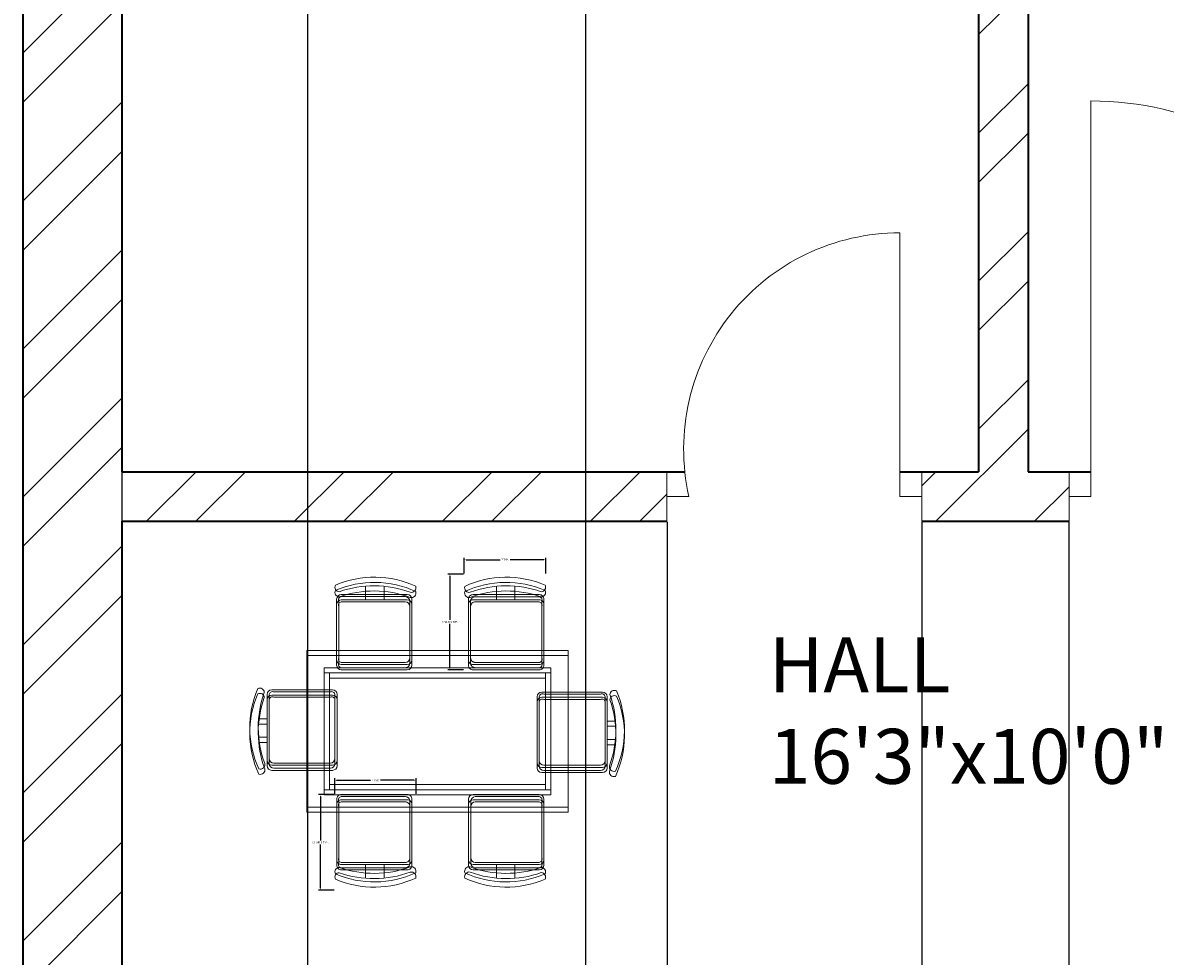
# Model space of a CAD drawing. Units: inches. Extents: x 2552 to 3217, y 1417 to 2737.
# Tile 21 of 25: x 2909 to 3013, y 2476 to 2561. Entities that reach past the tile are written whole.
import ezdxf

# ---------------------------------------------------------------- set-up
doc = ezdxf.new("R2010")
doc.units = ezdxf.units.IN
for name, color, linetype, lineweight in [('A-ANNO-DIMS', 2, 'Continuous', 18), ('A-AREA-IDEN', 7, 'Continuous', 18), ('A-DOOR', 21, 'Continuous', 18), ('A-FLOR-CASE', 9, 'Continuous', 18), ('A-FURN', 8, 'Continuous', 13), ('A-WALL', 7, 'Continuous', 35), ('A-WALL-PATT', 217, 'Continuous', 13)]:
    doc.layers.add(name, color=color, linetype=linetype, lineweight=lineweight)
doc.styles.get("Standard").update_dxf_attribs({"font": 'arial.ttf'})
doc.dimstyles.get("Standard").update_dxf_attribs({"dimtxt": 0.18, "dimasz": 0.18, "dimexe": 0.18, "dimexo": 0.0625, "dimgap": 0.09, "dimtad": 0, "dimtih": 1, "dimtoh": 1, "dimdec": 4, "dimzin": 0, "dimdsep": 46, "dimtxsty": 'Standard', "dimcen": 0.09, "dimadec": 0, "dimazin": 0, "dimtfac": 1, "dimtdec": 4, "dimtofl": 0, "dimtmove": 0, "dimatfit": 3, "dimfxl": 1, "dimtolj": 1, "dimtzin": 0, "dimarcsym": 0})

# ---------------------------------------------------------------- blocks, each defined once
blk = doc.blocks.new('TABLE-DINING-RECT')
for points in [[(0, 14.74), (23.77, 14.74), (23.77, 0.48), (0, 0.48)], [(0, 14.74), (23.77, 14.74), (23.77, 0.48), (0, 0.48)], [(0, 14.26), (23.77, 14.26), (23.77, 0), (0, 0)], [(0, 14.26), (23.77, 14.26), (23.77, 0), (0, 0)], [(1.58, 13.15), (22.19, 13.15), (22.19, 2.06), (1.58, 2.06)], [(1.58, 13.15), (22.19, 13.15), (22.19, 2.06), (1.58, 2.06)], [(1.58, 12.68), (22.19, 12.68), (22.19, 1.59), (1.58, 1.59)], [(1.58, 12.68), (22.19, 12.68), (22.19, 1.58), (1.58, 1.58)], [(2.06, 12.68), (21.71, 12.68), (21.71, 2.54), (2.06, 2.54)], [(2.06, 12.68), (21.71, 12.68), (21.71, 2.54), (2.06, 2.54)], [(2.06, 12.2), (21.71, 12.2), (21.71, 2.06), (2.06, 2.06)], [(2.06, 12.2), (21.71, 12.2), (21.71, 2.06), (2.06, 2.06)]]:
    blk.add_lwpolyline(points, close=True)
blk = doc.blocks.new('DINING-CHAIR-NORTH-EAST')
for points in [[(0.51, 7.05, -0.578392), (0.02, 7.59, -0.214524), (7.33, 7.69, -0.552014), (6.98, 7.1, 0.175809), (0.51, 7.05)], [(0.51, 7.05, -0.578392), (0.02, 7.59, -0.214524), (7.33, 7.69, -0.552014), (6.98, 7.1, 0.175809), (0.51, 7.05)], [(0.51, 6.58, -0.578392), (0.02, 7.12, -0.214524), (7.33, 7.22, -0.552014), (6.98, 6.63, 0.175809), (0.51, 6.58)], [(0.51, 6.58, -0.578392), (0.02, 7.12, -0.214524), (7.33, 7.22, -0.552014), (6.98, 6.63, 0.175809), (0.51, 6.58)], [(2.9, 6.84), (2.9, 7.6, 0.064759)], [(2.9, 6.84), (2.9, 7.6, 0.064759)], [(6.8, 6.84, -0.414214), (7.22, 6.42), (7.22, 0.9, -0.414214), (6.8, 0.48), (0.78, 0.48, -0.414214), (0.36, 0.9), (0.36, 6.42, -0.414214), (0.78, 6.84), (6.8, 6.84)], [(6.8, 6.84, -0.414214), (7.22, 6.42), (7.22, 0.9, -0.414214), (6.8, 0.48), (0.78, 0.48, -0.414214), (0.36, 0.9), (0.36, 6.42, -0.414214), (0.78, 6.84), (6.8, 6.84)], [(6.8, 6.37, -0.414214), (7.22, 5.95), (7.22, 0.42, -0.414214), (6.8, 0), (0.78, 0, -0.414214), (0.36, 0.42), (0.36, 5.95, -0.414214), (0.78, 6.37), (6.8, 6.37)], [(6.8, 6.37, -0.414214), (7.22, 5.95), (7.22, 0.42, -0.414214), (6.8, 0), (0.78, 0, -0.414214), (0.36, 0.42), (0.36, 5.95, -0.414214), (0.78, 6.37), (6.8, 6.37)], [(2.9, 6.37), (2.9, 7.13, 0.064759)], [(2.9, 6.37), (2.9, 7.13, 0.064759)]]:
    blk.add_lwpolyline(points, format="xyb")
for points in [[(4.58, 7.62), (4.58, 6.84)], [(4.58, 7.62), (4.58, 6.84)], [(4.58, 7.14), (4.58, 6.37)], [(4.58, 7.14), (4.58, 6.37)]]:
    blk.add_lwpolyline(points)
for points in [[(6.79, 6.65), (0.97, 6.65, 0.414214), (0.55, 6.23), (0.55, 1.09, 0.414214), (0.97, 0.67), (6.79, 0.67, 0.512069), (7.03, 1.09), (7.03, 6.23, 0.512069)], [(6.79, 6.65), (0.97, 6.65, 0.414214), (0.55, 6.23), (0.55, 1.09, 0.414214), (0.97, 0.66), (6.79, 0.66, 0.512069), (7.03, 1.09), (7.03, 6.23, 0.512069)], [(6.79, 6.18), (0.97, 6.18, 0.414214), (0.55, 5.76), (0.55, 0.61, 0.414214), (0.97, 0.19), (6.79, 0.19, 0.512069), (7.03, 0.61), (7.03, 5.76, 0.512069)], [(6.79, 6.18), (0.97, 6.18, 0.414214), (0.55, 5.76), (0.55, 0.61, 0.414214), (0.97, 0.19), (6.79, 0.19, 0.512069), (7.03, 0.61), (7.03, 5.76, 0.512069)]]:
    blk.add_lwpolyline(points, format="xyb", close=True)
blk = doc.blocks.new('DINING-CHAIR-SOUTH-WEST')
for points in [[(6.59, 2.06), (0.58, 2.06, -0.414214), (0.16, 2.48), (0.16, 8.01, -0.414214), (0.58, 8.43), (6.59, 8.43, -0.414214), (7.01, 8.01), (7.01, 2.48, -0.414214), (6.59, 2.06)], [(6.59, 2.06), (0.58, 2.06, -0.414214), (0.16, 2.48), (0.16, 8.01, -0.414214), (0.58, 8.43), (6.59, 8.43, -0.414214), (7.01, 8.01), (7.01, 2.48, -0.414214), (6.59, 2.06)], [(6.59, 1.58), (0.58, 1.58, -0.414214), (0.16, 2), (0.16, 7.53, -0.414214), (0.58, 7.95), (6.59, 7.95, -0.414214), (7.01, 7.53), (7.01, 2, -0.414214), (6.59, 1.58)], [(6.59, 1.58), (0.58, 1.58, -0.414214), (0.16, 2), (0.16, 7.53, -0.414214), (0.58, 7.95), (6.59, 7.95, -0.414214), (7.01, 7.53), (7.01, 2, -0.414214), (6.59, 1.58)], [(6.86, 1.85, -0.578392), (7.35, 1.31, -0.214524), (0.05, 1.21, -0.552014), (0.39, 1.8, 0.175809), (6.86, 1.85)], [(6.86, 1.85, -0.578392), (7.35, 1.31, -0.214524), (0.05, 1.21, -0.552014), (0.39, 1.8, 0.175809), (6.86, 1.85)], [(6.86, 1.37, -0.578392), (7.35, 0.83, -0.214524), (0.05, 0.74, -0.552014), (0.39, 1.32, 0.175809), (6.86, 1.37)], [(6.86, 1.37, -0.578392), (7.35, 0.83, -0.214524), (0.05, 0.74, -0.552014), (0.39, 1.32, 0.175809), (6.86, 1.37)], [(4.48, 2.06), (4.48, 1.3, 0.064759)], [(4.48, 2.06), (4.48, 1.3, 0.064759)], [(4.48, 1.58), (4.48, 0.82, 0.064759)], [(4.48, 1.58), (4.48, 0.82, 0.064759)]]:
    blk.add_lwpolyline(points, format="xyb")
for points in [[(0.58, 2.25), (6.4, 2.25, 0.414214), (6.82, 2.67), (6.82, 7.82, 0.414214), (6.4, 8.24), (0.58, 8.24, 0.512069), (0.35, 7.82), (0.35, 2.67, 0.512069)], [(0.58, 2.25), (6.4, 2.25, 0.414214), (6.82, 2.67), (6.82, 7.82, 0.414214), (6.4, 8.24), (0.58, 8.24, 0.512069), (0.35, 7.82), (0.35, 2.67, 0.512069)], [(0.58, 1.77), (6.4, 1.77, 0.414214), (6.82, 2.19), (6.82, 7.34, 0.414214), (6.4, 7.76), (0.58, 7.76, 0.512069), (0.35, 7.34), (0.35, 2.19, 0.512069)], [(0.58, 1.77), (6.4, 1.77, 0.414214), (6.82, 2.19), (6.82, 7.34, 0.414214), (6.4, 7.76), (0.58, 7.76, 0.512069), (0.35, 7.34), (0.35, 2.19, 0.512069)]]:
    blk.add_lwpolyline(points, format="xyb", close=True)
for points in [[(2.79, 1.28), (2.79, 2.06)], [(2.79, 1.28), (2.79, 2.06)], [(2.79, 0.81), (2.79, 1.58)], [(2.79, 0.81), (2.79, 1.58)]]:
    blk.add_lwpolyline(points)
blk = doc.blocks.new('*D35')
at = {"layer": 'A-ANNO-DIMS', "color": 0, "lineweight": -2, "transparency": 16777216}
for p, q in [((2948.98, 2511.21), (2947.55, 2511.21)), ((2947.73, 2511.03), (2947.73, 2507.04)), ((2947.73, 2502.68), (2947.73, 2506.67)), ((2948.98, 2502.5), (2947.55, 2502.5))]:
    blk.add_line(p, q, dxfattribs=at)
at = {"layer": 'A-ANNO-DIMS', "color": 0, "transparency": 16777216}
for points in [[(2947.7, 2511.03), (2947.76, 2511.03), (2947.73, 2511.21)], [(2947.7, 2502.68), (2947.76, 2502.68), (2947.73, 2502.5)]]:
    blk.add_solid(points, dxfattribs=at)
at = {"layer": 'Defpoints', "color": 0, "transparency": 16777216}
for p in [(2947.73, 2511.21), (2949.04, 2511.21), (2949.04, 2502.5)]:
    blk.add_point(p, dxfattribs=at)
at = {"layer": 'A-ANNO-DIMS', "color": 0, "transparency": 16777216, "insert": (2947.73, 2506.85), "char_height": 0.18, "attachment_point": 5}
blk.add_mtext('\\A1;CHAIR 9 TYP.', dxfattribs=at)
blk = doc.blocks.new('*D36')
at = {"layer": 'A-ANNO-DIMS', "color": 0, "lineweight": -2, "transparency": 16777216}
for p, q in [((2949.04, 2511.27), (2949.04, 2512.69)), ((2949.22, 2512.51), (2952.29, 2512.51)), ((2956.28, 2512.51), (2953.21, 2512.51)), ((2956.46, 2511.27), (2956.46, 2512.69))]:
    blk.add_line(p, q, dxfattribs=at)
at = {"layer": 'A-ANNO-DIMS', "color": 0, "transparency": 16777216}
for points in [[(2949.22, 2512.54), (2949.22, 2512.48), (2949.04, 2512.51)], [(2956.28, 2512.54), (2956.28, 2512.48), (2956.46, 2512.51)]]:
    blk.add_solid(points, dxfattribs=at)
at = {"layer": 'Defpoints', "color": 0, "transparency": 16777216}
for p in [(2956.46, 2512.51), (2949.04, 2511.21), (2956.46, 2511.21)]:
    blk.add_point(p, dxfattribs=at)
at = {"layer": 'A-ANNO-DIMS', "color": 0, "transparency": 16777216, "insert": (2952.75, 2512.51), "char_height": 0.18, "attachment_point": 5}
blk.add_mtext('\\A1;7 TYP.', dxfattribs=at)
blk = doc.blocks.new('*D41')
at = {"layer": 'A-ANNO-DIMS', "color": 0, "lineweight": -2, "transparency": 16777216}
for p, q in [((2937.18, 2491.14), (2935.76, 2491.14)), ((2935.94, 2490.96), (2935.94, 2486.97)), ((2935.94, 2482.62), (2935.94, 2486.61)), ((2937.18, 2482.44), (2935.76, 2482.44))]:
    blk.add_line(p, q, dxfattribs=at)
at = {"layer": 'A-ANNO-DIMS', "color": 0, "transparency": 16777216}
for points in [[(2935.91, 2490.96), (2935.97, 2490.96), (2935.94, 2491.14)], [(2935.91, 2482.62), (2935.97, 2482.62), (2935.94, 2482.44)]]:
    blk.add_solid(points, dxfattribs=at)
at = {"layer": 'Defpoints', "color": 0, "transparency": 16777216}
for p in [(2935.94, 2491.14), (2937.24, 2491.14), (2937.24, 2482.44)]:
    blk.add_point(p, dxfattribs=at)
at = {"layer": 'A-ANNO-DIMS', "color": 0, "transparency": 16777216, "insert": (2935.94, 2486.79), "char_height": 0.18, "attachment_point": 5}
blk.add_mtext('\\A1;CHAIR 9 TYP.', dxfattribs=at)
blk = doc.blocks.new('*D42')
at = {"layer": 'A-ANNO-DIMS', "color": 0, "lineweight": -2, "transparency": 16777216}
for p, q in [((2937.24, 2491.21), (2937.24, 2492.63)), ((2944.66, 2491.21), (2944.66, 2492.63)), ((2937.42, 2492.45), (2940.49, 2492.45)), ((2944.48, 2492.45), (2941.41, 2492.45))]:
    blk.add_line(p, q, dxfattribs=at)
at = {"layer": 'A-ANNO-DIMS', "color": 0, "transparency": 16777216}
for points in [[(2937.42, 2492.48), (2937.42, 2492.42), (2937.24, 2492.45)], [(2944.48, 2492.48), (2944.48, 2492.42), (2944.66, 2492.45)]]:
    blk.add_solid(points, dxfattribs=at)
at = {"layer": 'Defpoints', "color": 0, "transparency": 16777216}
for p in [(2944.66, 2492.45), (2937.24, 2491.14), (2944.66, 2491.14)]:
    blk.add_point(p, dxfattribs=at)
at = {"layer": 'A-ANNO-DIMS', "color": 0, "transparency": 16777216, "insert": (2940.95, 2492.45), "char_height": 0.18, "attachment_point": 5}
blk.add_mtext('\\A1;7 TYP.', dxfattribs=at)
blk = doc.blocks.new('*D56')
at = {"layer": 'A-ANNO-DIMS', "color": 0, "lineweight": -2, "transparency": 16777216}
for p, q in [((2967.49, 2515.95), (2967.49, 1482.53)), ((2990.69, 2515.95), (2990.69, 1482.53)), ((2967.67, 1482.71), (2978.76, 1482.71)), ((2990.51, 1482.71), (2979.41, 1482.71))]:
    blk.add_line(p, q, dxfattribs=at)
at = {"layer": 'A-ANNO-DIMS', "color": 0, "transparency": 16777216}
for points in [[(2967.67, 1482.74), (2967.67, 1482.68), (2967.49, 1482.71)], [(2990.51, 1482.74), (2990.51, 1482.68), (2990.69, 1482.71)]]:
    blk.add_solid(points, dxfattribs=at)
at = {"layer": 'Defpoints', "color": 0, "transparency": 16777216}
for p in [(2967.49, 2516.01), (2990.69, 2516.01), (2990.69, 1482.71)]:
    blk.add_point(p, dxfattribs=at)
at = {"layer": 'A-ANNO-DIMS', "color": 0, "transparency": 16777216, "insert": (2979.09, 1482.71), "char_height": 0.18, "attachment_point": 5}
blk.add_mtext('\\A1;23.2', dxfattribs=at)
blk = doc.blocks.new('*D57')
at = {"layer": 'A-ANNO-DIMS', "color": 0, "lineweight": -2, "transparency": 16777216}
for p, q in [((3004.08, 2515.95), (3004.08, 1482.53)), ((3036.34, 2515.95), (3036.34, 1482.53)), ((3004.26, 1482.71), (3019.75, 1482.71)), ((3036.16, 1482.71), (3020.68, 1482.71))]:
    blk.add_line(p, q, dxfattribs=at)
at = {"layer": 'A-ANNO-DIMS', "color": 0, "transparency": 16777216}
for points in [[(3004.26, 1482.74), (3004.26, 1482.68), (3004.08, 1482.71)], [(3036.16, 1482.74), (3036.16, 1482.68), (3036.34, 1482.71)]]:
    blk.add_solid(points, dxfattribs=at)
at = {"layer": 'Defpoints', "color": 0, "transparency": 16777216}
for p in [(3004.08, 2516.01), (3036.34, 2516.01), (3036.34, 1482.71)]:
    blk.add_point(p, dxfattribs=at)
at = {"layer": 'A-ANNO-DIMS', "color": 0, "transparency": 16777216, "insert": (3020.21, 1482.71), "char_height": 0.18, "attachment_point": 5}
blk.add_mtext('\\A1;32.255', dxfattribs=at)
blk = doc.blocks.new('*D64')
at = {"layer": 'A-ANNO-DIMS', "color": 0, "lineweight": -2, "transparency": 16777216}
for p, q in [((2646.35, 1551.58), (2646.35, 2709.49)), ((2646.53, 2709.31), (2802.77, 2709.31)), ((2959.93, 2709.31), (2803.69, 2709.31)), ((2960.11, 1551.58), (2960.11, 2709.49))]:
    blk.add_line(p, q, dxfattribs=at)
at = {"layer": 'A-ANNO-DIMS', "color": 0, "transparency": 16777216}
for points in [[(2646.53, 2709.34), (2646.53, 2709.28), (2646.35, 2709.31)], [(2959.93, 2709.34), (2959.93, 2709.28), (2960.11, 2709.31)]]:
    blk.add_solid(points, dxfattribs=at)
at = {"layer": 'Defpoints', "color": 0, "transparency": 16777216}
for p in [(2960.11, 2709.31), (2646.35, 1551.51), (2960.11, 1551.51)]:
    blk.add_point(p, dxfattribs=at)
at = {"layer": 'A-ANNO-DIMS', "color": 0, "transparency": 16777216, "insert": (2803.23, 2709.31), "char_height": 0.18, "attachment_point": 5}
blk.add_mtext('\\A1;313.76', dxfattribs=at)
blk = doc.blocks.new('*D67')
at = {"layer": 'A-ANNO-DIMS', "color": 0, "lineweight": -2, "transparency": 16777216}
for p, q in [((2917.85, 2640.45), (2917.85, 1482.53)), ((2934.77, 2624.73), (2934.77, 1482.53)), ((2918.03, 1482.71), (2925.86, 1482.71)), ((2934.59, 1482.71), (2926.76, 1482.71))]:
    blk.add_line(p, q, dxfattribs=at)
at = {"layer": 'A-ANNO-DIMS', "color": 0, "transparency": 16777216}
for points in [[(2918.03, 1482.74), (2918.03, 1482.68), (2917.85, 1482.71)], [(2934.59, 1482.74), (2934.59, 1482.68), (2934.77, 1482.71)]]:
    blk.add_solid(points, dxfattribs=at)
at = {"layer": 'Defpoints', "color": 0, "transparency": 16777216}
for p in [(2917.85, 2640.51), (2934.77, 2624.79), (2934.77, 1482.71)]:
    blk.add_point(p, dxfattribs=at)
at = {"layer": 'A-ANNO-DIMS', "color": 0, "transparency": 16777216, "insert": (2926.31, 1482.71), "char_height": 0.18, "attachment_point": 5}
blk.add_mtext('\\A1;16.912', dxfattribs=at)

msp = doc.modelspace()

# ---------------------------------------------------------------- hatches: boundary and pattern name
at = {"layer": 'A-WALL-PATT'}
h = msp.add_hatch(dxfattribs=at)
h.set_pattern_fill('ANSI32', color=256)
h.paths.add_polyline_path([(2756.676, 2649.5125), (2637.3535, 2649.5125), (2637.3535, 2617.9626), (2641.8535, 2617.9626), (2646.3535, 2617.9626), (2646.3535, 2640.5125), (2724.3535, 2640.5125), (2724.3535, 2520.5125), (2720.299, 2520.5125), (2720.299, 2516.0125), (2733.4075, 2516.0125), (2733.4075, 2518.2213), (2733.4075, 2520.5125), (2728.8535, 2520.5125), (2728.8535, 2640.5125), (2756.676, 2640.5125)])
h.paths.add_polyline_path([(2848.8535, 2649.5125), (2804.676, 2649.5125), (2804.676, 2640.5125), (2839.8535, 2640.5125), (2839.8535, 2598.3517), (2848.8535, 2598.3517)])
h.paths.add_polyline_path([(2646.3535, 2516.0125), (2697.9593, 2516.0125), (2697.9593, 2518.2625), (2697.9593, 2520.5125), (2646.3535, 2520.5125), (2646.3535, 2581.9626), (2637.3535, 2581.9626), (2637.3535, 2364.3298), (2646.3535, 2364.3298), (2646.3535, 2387.0125), (2724.3535, 2387.0125), (2724.3535, 2267.0125), (2721.0443, 2267.0125), (2721.0443, 2262.5125), (2733.7854, 2262.5125), (2733.7854, 2264.7625), (2733.7854, 2267.0125), (2728.8535, 2267.0125), (2728.8535, 2387.0125), (2839.8535, 2387.0125), (2839.8535, 2363.8387), (2848.8535, 2363.8387), (2848.8535, 2403.7415), (2844.3535, 2403.7415), (2839.8535, 2403.7415), (2839.8535, 2396.0125), (2646.3535, 2396.0125)])
h.paths.add_polyline_path([(2848.8535, 2550.3517), (2844.3535, 2550.3517), (2839.8535, 2550.3517), (2839.8535, 2520.5125), (2801.9195, 2520.5125), (2801.9195, 2518.2625), (2801.9195, 2516.0125), (2839.8535, 2516.0125), (2839.8535, 2507.5813), (2848.8535, 2507.5813)], flags=17)
h.paths.add_polyline_path([(2848.8535, 2483.5813), (2844.3535, 2483.5813), (2839.8535, 2483.5813), (2839.8535, 2468.0125), (2773.8535, 2468.0125), (2773.8535, 2516.0125), (2778.1336, 2516.0125), (2778.1336, 2520.5125), (2766.696, 2520.5125), (2766.696, 2518.2625), (2766.696, 2516.0125), (2769.3535, 2516.0125), (2769.3535, 2463.5125), (2839.8535, 2463.5125), (2839.8535, 2431.0782), (2848.8535, 2431.0782)], flags=17)
h.paths.add_polyline_path([(2917.8535, 2569.2764), (2913.3535, 2569.2764), (2908.8535, 2569.2764), (2908.8535, 2433.001), (2917.8535, 2433.001), (2917.8535, 2516.0125), (2967.486, 2516.0125), (2967.486, 2520.5125), (2917.8535, 2520.5125)])
h.paths.add_polyline_path([(3000.3535, 2640.5125), (2995.8535, 2640.5125), (2995.8535, 2520.5125), (2990.688, 2520.5125), (2990.688, 2516.0125), (3004.0844, 2516.0125), (3004.0844, 2518.2625), (3004.0844, 2520.5125), (3000.3535, 2520.5125)])
h.paths.add_polyline_path([(3120.3535, 2561.3689), (3115.8535, 2561.3689), (3111.3535, 2561.3689), (3111.3535, 2520.5125), (3070.9814, 2520.5125), (3070.9814, 2518.2625), (3070.9814, 2516.0125), (3111.3535, 2516.0125), (3111.3535, 2505.1841), (3120.3535, 2505.1841)])
h.paths.add_polyline_path([(3120.3535, 2481.1841), (3115.8535, 2481.1841), (3111.3535, 2481.1841), (3111.3535, 2468.0125), (3045.3535, 2468.0125), (3045.3535, 2516.0125), (3048.9787, 2516.0125), (3048.9787, 2520.5125), (3036.3395, 2520.5125), (3036.3395, 2516.0125), (3040.8535, 2516.0125), (3040.8535, 2463.5125), (3111.3535, 2463.5125), (3111.3535, 2396.0125), (2917.8535, 2396.0125), (2917.8535, 2403.4124), (2913.3535, 2403.4124), (2908.8535, 2403.4124), (2908.8535, 2182.5756), (2917.8535, 2182.5756), (2917.8535, 2262.5125), (2968.001, 2262.5125), (2968.001, 2264.7625), (2968.001, 2267.0125), (2917.8535, 2267.0125), (2917.8535, 2387.0125), (3111.3535, 2387.0125), (3111.3535, 2352.2435), (3120.3535, 2352.2435)])
h.paths.add_polyline_path([(3120.3535, 2304.2435), (3115.8535, 2304.2435), (3111.3535, 2304.2435), (3111.3535, 2267.0125), (3073.8616, 2267.0125), (3073.8616, 2264.7625), (3073.8616, 2262.5125), (3111.3535, 2262.5125), (3111.3535, 2252.376), (3120.3535, 2252.376)], flags=17)
h.paths.add_polyline_path([(3120.3535, 2228.376), (3115.8535, 2228.376), (3111.3535, 2228.376), (3111.3535, 2214.5125), (3045.3535, 2214.5125), (3045.3535, 2262.5125), (3049.3096, 2262.5125), (3049.3096, 2267.0125), (3035.0125, 2267.0125), (3035.0125, 2262.5125), (3040.8535, 2262.5125), (3040.8535, 2210.0125), (3111.3535, 2210.0125), (3111.3535, 2142.5125), (2917.8535, 2142.5125), (2917.8535, 2150.2408), (2913.3535, 2150.2408), (2908.8535, 2150.2408), (2908.8535, 1924.9905), (2917.8535, 1924.9905), (2917.8535, 2009.0125), (2971.959, 2009.0125), (2971.959, 2011.2625), (2971.959, 2013.5125), (2917.8535, 2013.5125), (2917.8535, 2133.5125), (2995.8535, 2133.5125), (2995.8535, 2013.5125), (2992.1797, 2013.5125), (2992.1797, 2009.0125), (3004.3344, 2009.0125), (3004.3344, 2011.2625), (3004.3344, 2013.5125), (3000.3535, 2013.5125), (3000.3535, 2133.5125), (3111.3535, 2133.5125), (3111.3535, 2115.0291), (3120.3535, 2115.0291)])
h.paths.add_polyline_path([(3000.3535, 2387.0125), (2995.8535, 2387.0125), (2995.8535, 2267.0125), (2991.3326, 2267.0125), (2991.3326, 2262.5125), (3004.1044, 2262.5125), (3004.1044, 2264.7625), (3004.1044, 2267.0125), (3000.3535, 2267.0125)], flags=17)
h.paths.add_polyline_path([(3120.3535, 1973.2388), (3115.8535, 1973.2388), (3111.3535, 1973.2388), (3111.3535, 1961.0125), (3045.3535, 1961.0125), (3045.3535, 2009.0125), (3048.9101, 2009.0125), (3048.9101, 2013.5125), (3037.105, 2013.5125), (3037.105, 2011.2625), (3037.105, 2009.0125), (3040.8535, 2009.0125), (3040.8535, 1956.5125), (3111.3535, 1956.5125), (3111.3535, 1889.0125), (2917.8535, 1889.0125), (2917.8535, 1895.7215), (2913.3535, 1895.7215), (2908.8535, 1895.7215), (2908.8535, 1844.2217), (2917.8535, 1844.2217), (2917.8535, 1880.0125), (3111.3535, 1880.0125), (3111.3535, 1846.9541), (3120.3535, 1846.9541)])
h.paths.add_polyline_path([(3120.3535, 2067.0291), (3111.3535, 2067.0291), (3111.3535, 2013.5125), (3071.3001, 2013.5125), (3071.3001, 2009.0125), (3111.3535, 2009.0125), (3111.3535, 1997.2388), (3120.3535, 1997.2388)], flags=0)
h.paths.add_polyline_path([(3120.3535, 1798.9541), (3115.8535, 1798.9541), (3111.3535, 1798.9541), (3111.3535, 1760.0125), (3071.2497, 1760.0125), (3071.2497, 1757.7625), (3071.2497, 1755.5125), (3111.3535, 1755.5125), (3111.3535, 1746.162), (3120.3535, 1746.2478)])
h.paths.add_polyline_path([(3120.3535, 1722.2049), (3111.3535, 1722.2049), (3111.3535, 1707.5125), (3045.3535, 1707.5125), (3045.3535, 1755.5125), (3048.6624, 1755.5125), (3048.6624, 1760.0125), (3035.3703, 1760.0125), (3035.3703, 1755.5125), (3040.8535, 1755.5125), (3040.8535, 1703.0125), (3111.3535, 1703.0125), (3111.3535, 1635.5125), (2917.8535, 1635.5125), (2917.8535, 1643.1366), (2913.3535, 1643.1366), (2908.8535, 1643.1366), (2908.8535, 1626.5125), (3120.3535, 1626.5125)])
h.paths.add_polyline_path([(2917.8535, 1755.5125), (2973.2287, 1755.5125), (2973.2287, 1757.7625), (2973.2287, 1760.0125), (2917.8535, 1760.0125), (2917.8535, 1808.2217), (2913.3535, 1808.2217), (2908.8535, 1808.2217), (2908.8535, 1676.1665), (2917.8535, 1676.1665)])
h.paths.add_polyline_path([(3000.3535, 1880.0125), (2995.8535, 1880.0125), (2995.8535, 1760.0125), (2992.9329, 1760.0125), (2992.9329, 1755.5125), (3003.8766, 1755.5125), (3003.8766, 1757.7625), (3003.8766, 1760.0125), (3000.3535, 1760.0125)])
h.paths.add_polyline_path([(2848.8535, 1896.6971), (2844.3535, 1896.6971), (2839.8535, 1896.6971), (2839.8535, 1889.0125), (2646.3535, 1889.0125), (2646.3535, 2009.0125), (2700.5253, 2009.0125), (2700.5253, 2011.2625), (2700.5253, 2013.5125), (2646.3535, 2013.5125), (2646.3535, 2053.1812), (2641.8535, 2053.1812), (2637.3535, 2053.1812), (2637.3535, 1836.254), (2646.3535, 1836.254), (2646.3535, 1880.0125), (2724.3535, 1880.0125), (2724.3535, 1760.0125), (2721.2473, 1760.0125), (2721.2473, 1755.5125), (2731.9187, 1755.5125), (2731.9187, 1757.7625), (2731.9187, 1760.0125), (2728.8535, 1760.0125), (2728.8535, 1880.0125), (2839.8535, 1880.0125), (2839.8535, 1840.3813), (2848.8535, 1840.3813)])
h.paths.add_polyline_path([(2848.8535, 1792.3813), (2844.3535, 1792.3813), (2839.8535, 1792.3813), (2839.8535, 1760.0125), (2797.8845, 1760.0125), (2797.8845, 1755.5125), (2839.8535, 1755.5125), (2839.8535, 1743.3688), (2844.3535, 1743.3688), (2848.8535, 1743.3688)], flags=0)
h.paths.add_polyline_path([(2848.8535, 1719.3688), (2844.3535, 1719.3688), (2839.8535, 1719.3688), (2839.8535, 1707.5125), (2773.8535, 1707.5125), (2773.8535, 1755.5125), (2777.716, 1755.5125), (2777.716, 1760.0125), (2760.9247, 1760.0125), (2760.9247, 1757.9721), (2760.9247, 1755.5125), (2769.3535, 1755.5125), (2769.3535, 1703.0125), (2839.8535, 1703.0125), (2839.8535, 1673.0277), (2848.8535, 1672.9407)], flags=0)
h.paths.add_polyline_path([(2646.3535, 1755.5125), (2702.9171, 1755.5125), (2702.9171, 1757.7625), (2702.9171, 1760.0125), (2646.3535, 1760.0125), (2646.3535, 1800.254), (2641.8535, 1800.254), (2637.3535, 1800.254), (2637.3535, 1626.5125), (2848.8535, 1626.5125), (2848.8535, 1643.1187), (2844.3535, 1643.1187), (2839.8535, 1643.1187), (2839.8535, 1635.5125), (2646.3535, 1635.5125)])
h.paths.add_polyline_path([(2848.8535, 2148.8427), (2844.3535, 2148.8427), (2839.8535, 2148.8427), (2839.8535, 2142.5125), (2646.3535, 2142.5125), (2646.3535, 2262.5125), (2701.3562, 2262.5125), (2701.3562, 2264.7625), (2701.3562, 2267.0125), (2646.3535, 2267.0125), (2646.3535, 2328.3298), (2637.3535, 2328.3298), (2637.3535, 2089.1812), (2646.3535, 2089.1812), (2646.3535, 2133.5125), (2839.8535, 2133.5125), (2839.8535, 2097.5966), (2848.8535, 2097.5966)])
h.paths.add_polyline_path([(2728.8535, 2133.5125), (2724.3535, 2133.5125), (2724.3535, 2013.5125), (2719.6039, 2013.5125), (2719.6039, 2009.0125), (2732.5784, 2009.0125), (2732.5784, 2011.2625), (2732.5784, 2013.5125), (2728.8535, 2013.5125)])
h.paths.add_polyline_path([(2848.8535, 1970.0557), (2844.3535, 1970.0557), (2839.8535, 1970.0557), (2839.8535, 1961.0125), (2773.8535, 1961.0125), (2773.8535, 2009.0125), (2777.3388, 2009.0125), (2777.3388, 2013.5125), (2764.7681, 2013.5125), (2764.7681, 2009.0125), (2769.3535, 2009.0125), (2769.3535, 1956.5125), (2839.8535, 1956.5125), (2839.8535, 1924.7199), (2848.8535, 1924.7199)], flags=17)
h.paths.add_polyline_path([(2848.8535, 2049.5966), (2844.3535, 2049.5966), (2839.8535, 2049.5966), (2839.8535, 2013.5125), (2798.198, 2013.5125), (2798.198, 2011.2625), (2798.198, 2009.0125), (2839.8535, 2009.0125), (2839.8535, 1994.0557), (2848.8535, 1994.0557)], flags=17)
h.paths.add_polyline_path([(2848.8535, 2315.8387), (2839.8535, 2315.8387), (2839.8535, 2267.0125), (2799.3375, 2267.0125), (2799.3375, 2264.7625), (2799.3375, 2262.5125), (2839.8535, 2262.5125), (2839.8535, 2253.2843), (2848.8535, 2253.2843)], flags=17)
h.paths.add_polyline_path([(2848.8535, 2229.2843), (2839.8535, 2229.2843), (2839.8535, 2177.6936), (2848.8535, 2177.6936)], flags=17)
h.paths.add_polyline_path([(2839.8535, 2214.5125), (2773.8535, 2214.5125), (2773.8535, 2262.5125), (2777.6984, 2262.5125), (2777.6984, 2267.0125), (2763.8226, 2267.0125), (2763.8226, 2262.5125), (2769.3535, 2262.5125), (2769.3535, 2210.0125), (2839.8535, 2210.0125)], flags=17)
h.paths.add_polyline_path([(3050.32, 2520.2817), (3088.9114, 2520.2817), (3088.9114, 2538.939), (3050.32, 2538.939)], flags=9)

# ---------------------------------------------------------------- linework, layer by layer
at = {"layer": 'A-DOOR'}
for p, q in [((3006.0844, 2518.2625), (3006.0844, 2554.2625)), ((2988.688, 2518.2625), (2988.688, 2542.2625)), ((2967.486, 2516.0125), (2967.486, 2520.5125)), ((2967.486, 2520.5125), (2967.486, 2518.2625)), ((2990.688, 2520.5125), (2990.688, 2516.0125)), ((3004.0844, 2520.5125), (3004.0844, 2516.0125)), ((2967.486, 2518.2625), (2969.486, 2518.2625)), ((2990.688, 2518.2625), (2988.688, 2518.2625)), ((2990.688, 2516.0125), (2990.688, 2518.2625)), ((3004.0844, 2516.0125), (3004.0844, 2518.2625)), ((3004.0844, 2518.2625), (3006.0844, 2518.2625))]:
    msp.add_line(p, q, dxfattribs=at)
for centre, radius, start, end in [((3006.0844, 2525.1743), 29.0882, 346.25422, 90), ((2988.688, 2522.5809), 19.6816, 90, 192.674554)]:
    msp.add_arc(centre, radius, start, end, dxfattribs=at)
at = {"layer": 'A-FLOR-CASE'}
msp.add_line((2934.7654, 2520.5125), (2934.7654, 2624.7942), dxfattribs=at)
at = {"layer": 'A-FURN'}
for points in [[(2937.6502, 2509.6032, -0.17580919), (2944.1246, 2509.5542, 0.57839206), (2944.6151, 2510.0935, 0.21452438), (2937.3068, 2510.1916, 0.55201397), (2937.6502, 2509.6032, -0.06507904)], [(2937.6502, 2509.603, -0.17580919), (2944.1246, 2509.5539, 0.57839206), (2944.6151, 2510.0933, 0.21452438), (2937.3068, 2510.1913, 0.55201397), (2937.6502, 2509.603, -0.06507904)], [(2937.6502, 2509.1278, -0.17580919), (2944.1246, 2509.0788, 0.57839206), (2944.6151, 2509.6181, 0.21452438), (2937.3068, 2509.7162, 0.55201397), (2937.6502, 2509.1278, -0.06507904)], [(2937.6502, 2509.1276, -0.17580919), (2944.1246, 2509.0785, 0.57839206), (2944.6151, 2509.6179, 0.21452438), (2937.3068, 2509.7159, 0.55201397), (2937.6502, 2509.1276, -0.06507904)], [(2943.8499, 2509.3434), (2937.8393, 2509.3434, 0.41421356), (2937.4188, 2508.9228), (2937.4188, 2503.3962, 0.41421356), (2937.8393, 2502.9756), (2943.8499, 2502.9756, 0.41421356), (2944.2704, 2503.3962), (2944.2704, 2508.9228, 0.41421356), (2943.8499, 2509.3434)], [(2943.8499, 2509.3431), (2937.8393, 2509.3431, 0.41421356), (2937.4188, 2508.9226), (2937.4188, 2503.3959, 0.41421356), (2937.8393, 2502.9754), (2943.8499, 2502.9754, 0.41421356), (2944.2704, 2503.3959), (2944.2704, 2508.9226, 0.41421356), (2943.8499, 2509.3431)], [(2941.7387, 2509.3434), (2941.7387, 2510.1035, -0.06475861)], [(2941.7387, 2509.3431), (2941.7387, 2510.1033, -0.06475861)], [(2941.7387, 2508.8679), (2941.7387, 2509.6281, -0.06475861)], [(2941.7387, 2508.8677), (2941.7387, 2509.6279, -0.06475861)], [(2943.8499, 2508.8679), (2937.8393, 2508.8679, 0.41421356), (2937.4188, 2508.4474), (2937.4188, 2502.9207, 0.41421356), (2937.8393, 2502.5002), (2943.8499, 2502.5002, 0.41421356), (2944.2704, 2502.9207), (2944.2704, 2508.4474, 0.41421356), (2943.8499, 2508.8679)], [(2943.8499, 2508.8677), (2937.8393, 2508.8677, 0.41421356), (2937.4188, 2508.4472), (2937.4188, 2502.9205, 0.41421356), (2937.8393, 2502.5), (2943.8499, 2502.5, 0.41421356), (2944.2704, 2502.9205), (2944.2704, 2508.4472, 0.41421356), (2943.8499, 2508.8677)], [(2930.8766, 2493.9684, -0.57839206), (2930.3373, 2493.4779, -0.21452438), (2930.2392, 2500.7862, -0.55201397), (2930.8276, 2500.4428, 0.17580937), (2930.8766, 2493.9684)], [(2930.8767, 2493.9681, -0.57839206), (2930.3373, 2493.4777, -0.21452438), (2930.2393, 2500.7859, -0.55201397), (2930.8276, 2500.4426, 0.17580937), (2930.8767, 2493.9681)], [(2930.8766, 2493.493, -0.57839206), (2930.3373, 2493.0025, -0.21452438), (2930.2392, 2500.3108, -0.55201397), (2930.8276, 2499.9674, 0.17580937), (2930.8766, 2493.493)], [(2930.8767, 2493.4927, -0.57839206), (2930.3373, 2493.0022, -0.21452438), (2930.2393, 2500.3105, -0.55201397), (2930.8276, 2499.9672, 0.17580937), (2930.8767, 2493.4927)], [(2931.0875, 2500.2537, -0.41421356), (2931.508, 2500.6743), (2937.0347, 2500.6743, -0.41421356), (2937.4552, 2500.2537), (2937.4552, 2494.2431, -0.41421356), (2937.0347, 2493.8226), (2931.508, 2493.8226, -0.41421356), (2931.0875, 2494.2431), (2931.0875, 2500.2537)], [(2931.0875, 2500.2535, -0.41421356), (2931.508, 2500.674), (2937.0347, 2500.674, -0.41421356), (2937.4552, 2500.2535), (2937.4552, 2494.2428, -0.41421356), (2937.0347, 2493.8223), (2931.508, 2493.8223, -0.41421356), (2931.0875, 2494.2428), (2931.0875, 2500.2535)], [(2931.0875, 2499.7783, -0.41421356), (2931.508, 2500.1988), (2937.0347, 2500.1988, -0.41421356), (2937.4552, 2499.7783), (2937.4552, 2493.7677, -0.41421356), (2937.0347, 2493.3472), (2931.508, 2493.3472, -0.41421356), (2931.0875, 2493.7677), (2931.0875, 2499.7783)], [(2931.0875, 2499.7781, -0.41421356), (2931.508, 2500.1986), (2937.0347, 2500.1986, -0.41421356), (2937.4552, 2499.7781), (2937.4552, 2493.7674, -0.41421356), (2937.0347, 2493.3469), (2931.508, 2493.3469, -0.41421356), (2931.0875, 2493.7674), (2931.0875, 2499.7781)], [(2962.0396, 2500.0479, 0.41421356), (2961.619, 2500.4684), (2956.0924, 2500.4684, 0.41421356), (2955.6718, 2500.0479), (2955.6718, 2494.0372, 0.41421356), (2956.0924, 2493.6167), (2961.619, 2493.6167, 0.41421356), (2962.0396, 2494.0372), (2962.0396, 2500.0479)], [(2962.0396, 2499.5725, 0.41421356), (2961.619, 2499.993), (2956.0924, 2499.993, 0.41421356), (2955.6718, 2499.5725), (2955.6718, 2493.5618, 0.41421356), (2956.0924, 2493.1413), (2961.619, 2493.1413, 0.41421356), (2962.0396, 2493.5618), (2962.0396, 2499.5725)], [(2962.0396, 2500.0476, 0.41421356), (2961.6191, 2500.4682), (2956.0924, 2500.4682, 0.41421356), (2955.6719, 2500.0476), (2955.6719, 2494.037, 0.41421356), (2956.0924, 2493.6165), (2961.6191, 2493.6165, 0.41421356), (2962.0396, 2494.037), (2962.0396, 2500.0476)], [(2962.0396, 2499.5722, 0.41421356), (2961.6191, 2499.9927), (2956.0924, 2499.9927, 0.41421356), (2955.6719, 2499.5722), (2955.6719, 2493.5616, 0.41421356), (2956.0924, 2493.1411), (2961.6191, 2493.1411, 0.41421356), (2962.0396, 2493.5616), (2962.0396, 2499.5722)], [(2962.2994, 2500.237, -0.17580919), (2962.2504, 2493.7625, 0.57839206), (2962.7897, 2493.2721, 0.21452438), (2962.8878, 2500.5803, 0.55201397), (2962.2994, 2500.237, -0.06507904)], [(2962.2994, 2500.2367, -0.17580919), (2962.2504, 2493.7623, 0.57839206), (2962.7897, 2493.2718, 0.21452438), (2962.8878, 2500.5801, 0.55201397), (2962.2994, 2500.2367, -0.06507904)], [(2962.2994, 2499.7616, -0.17580919), (2962.2504, 2493.2871, 0.57839206), (2962.7897, 2492.7966, 0.21452438), (2962.8878, 2500.1049, 0.55201397), (2962.2994, 2499.7616, -0.06507904)], [(2962.2994, 2499.7613, -0.17580919), (2962.2504, 2493.2869, 0.57839206), (2962.7897, 2492.7964, 0.21452438), (2962.8878, 2500.1047, 0.55201397), (2962.2994, 2499.7613, -0.06507904)], [(2931.0875, 2496.3543), (2930.3273, 2496.3543, 0.06475861)], [(2931.0875, 2496.3541), (2930.3273, 2496.3541, 0.06475861)], [(2931.0875, 2495.8789), (2930.3273, 2495.8789, 0.06475861)], [(2931.0875, 2495.8787), (2930.3273, 2495.8787, 0.06475861)], [(2962.0396, 2496.1485), (2962.7997, 2496.1485, -0.06475861)], [(2962.0396, 2496.1482), (2962.7997, 2496.1482, -0.06475861)], [(2962.0396, 2495.6731), (2962.7997, 2495.6731, -0.06475861)], [(2962.0396, 2495.6728), (2962.7997, 2495.6728, -0.06475861)], [(2955.8606, 2484.7759, 0.41421356), (2956.2811, 2485.1964), (2956.2811, 2490.7231, 0.41421356), (2955.8606, 2491.1436), (2949.8499, 2491.1436, 0.41421356), (2949.4294, 2490.7231), (2949.4294, 2485.1964, 0.41421356), (2949.8499, 2484.7759), (2955.8606, 2484.7759)], [(2955.8606, 2484.7756, 0.41421356), (2956.2811, 2485.1961), (2956.2811, 2490.7228, 0.41421356), (2955.8606, 2491.1433), (2949.85, 2491.1433, 0.41421356), (2949.4294, 2490.7228), (2949.4294, 2485.1961, 0.41421356), (2949.85, 2484.7756), (2955.8606, 2484.7756)], [(2955.8606, 2484.3005, 0.41421356), (2956.2811, 2484.721), (2956.2811, 2490.2477, 0.41421356), (2955.8606, 2490.6682), (2949.8499, 2490.6682, 0.41421356), (2949.4294, 2490.2477), (2949.4294, 2484.721, 0.41421356), (2949.8499, 2484.3005), (2955.8606, 2484.3005)], [(2955.8606, 2484.3002, 0.41421356), (2956.2811, 2484.7207), (2956.2811, 2490.2474, 0.41421356), (2955.8606, 2490.6679), (2949.85, 2490.6679, 0.41421356), (2949.4294, 2490.2474), (2949.4294, 2484.7207, 0.41421356), (2949.85, 2484.3002), (2955.8606, 2484.3002)], [(2956.0497, 2484.516, -0.17580928), (2949.5753, 2484.5651, 0.57839206), (2949.0848, 2484.0257, 0.21452438), (2956.3931, 2483.9277, 0.55201397), (2956.0497, 2484.516, -0.06507904)], [(2956.0497, 2484.5158, -0.17580928), (2949.5753, 2484.5648, 0.57839206), (2949.0848, 2484.0255, 0.21452438), (2956.3931, 2483.9274, 0.55201397), (2956.0497, 2484.5158, -0.06507904)], [(2951.9612, 2484.7759), (2951.9612, 2484.0157, -0.06475861)], [(2951.9612, 2484.7756), (2951.9612, 2484.0155, -0.06475861)], [(2951.9612, 2484.3005), (2951.9612, 2483.5403, -0.06475861)], [(2951.9612, 2484.3002), (2951.9612, 2483.5401, -0.06475861)], [(2956.0497, 2484.0406, -0.17580928), (2949.5753, 2484.0896, 0.57839206), (2949.0848, 2483.5503, 0.21452438), (2956.3931, 2483.4523, 0.55201397), (2956.0497, 2484.0406, -0.06507904)], [(2956.0497, 2484.0404, -0.17580928), (2949.5753, 2484.0894, 0.57839206), (2949.0848, 2483.5501, 0.21452438), (2956.3931, 2483.452, 0.55201397), (2956.0497, 2484.0404, -0.06507904)]]:
    msp.add_lwpolyline(points, format="xyb", dxfattribs=at)
for points in [[(2937.8418, 2509.1539), (2943.6605, 2509.1539, -0.41421356), (2944.081, 2508.7334), (2944.081, 2503.5856, -0.41421356), (2943.6605, 2503.1651), (2937.8418, 2503.1651, -0.51206948), (2937.6082, 2503.5856), (2937.6082, 2508.7334, -0.51206948)], [(2937.8418, 2509.1537), (2943.6605, 2509.1537, -0.41421356), (2944.081, 2508.7332), (2944.081, 2503.5854, -0.41421356), (2943.6605, 2503.1648), (2937.8418, 2503.1648, -0.51206948), (2937.6082, 2503.5854), (2937.6082, 2508.7332, -0.51206948)], [(2937.8418, 2508.6785), (2943.6605, 2508.6785, -0.41421356), (2944.081, 2508.258), (2944.081, 2503.1102, -0.41421356), (2943.6605, 2502.6897), (2937.8418, 2502.6897, -0.51206948), (2937.6082, 2503.1102), (2937.6082, 2508.258, -0.51206948)], [(2937.8418, 2508.6783), (2943.6605, 2508.6783, -0.41421356), (2944.081, 2508.2577), (2944.081, 2503.1099, -0.41421356), (2943.6605, 2502.6894), (2937.8418, 2502.6894, -0.51206948), (2937.6082, 2503.1099), (2937.6082, 2508.2577, -0.51206948)], [(2931.2769, 2500.2512), (2931.2769, 2494.4325, 0.41421356), (2931.6974, 2494.012), (2936.8452, 2494.012, 0.41421356), (2937.2657, 2494.4325), (2937.2657, 2500.2512, 0.51206948), (2936.8452, 2500.4848), (2931.6974, 2500.4848, 0.51206948)], [(2931.2769, 2500.2509), (2931.2769, 2494.4323, 0.41421356), (2931.6974, 2494.0118), (2936.8452, 2494.0118, 0.41421356), (2937.2657, 2494.4323), (2937.2657, 2500.2509, 0.51206948), (2936.8452, 2500.4846), (2931.6974, 2500.4846, 0.51206948)], [(2931.2769, 2499.7758), (2931.2769, 2493.9571, 0.41421356), (2931.6974, 2493.5366), (2936.8452, 2493.5366, 0.41421356), (2937.2657, 2493.9571), (2937.2657, 2499.7758, 0.51206948), (2936.8452, 2500.0094), (2931.6974, 2500.0094, 0.51206948)], [(2931.2769, 2499.7755), (2931.2769, 2493.9569, 0.41421356), (2931.6974, 2493.5363), (2936.8452, 2493.5363, 0.41421356), (2937.2657, 2493.9569), (2937.2657, 2499.7755, 0.51206948), (2936.8452, 2500.0091), (2931.6974, 2500.0091, 0.51206948)], [(2961.8501, 2500.0453), (2961.8501, 2494.2267, -0.41421356), (2961.4296, 2493.8062), (2956.2818, 2493.8062, -0.41421356), (2955.8613, 2494.2267), (2955.8613, 2500.0453, -0.51206948), (2956.2818, 2500.279), (2961.4296, 2500.279, -0.51206948)], [(2961.8501, 2500.0451), (2961.8501, 2494.2264, -0.41421356), (2961.4296, 2493.8059), (2956.2818, 2493.8059, -0.41421356), (2955.8613, 2494.2264), (2955.8613, 2500.0451, -0.51206948), (2956.2818, 2500.2787), (2961.4296, 2500.2787, -0.51206948)], [(2961.8501, 2499.5699), (2961.8501, 2493.7513, -0.41421356), (2961.4296, 2493.3307), (2956.2818, 2493.3307, -0.41421356), (2955.8613, 2493.7513), (2955.8613, 2499.5699, -0.51206948), (2956.2818, 2499.8035), (2961.4296, 2499.8035, -0.51206948)], [(2961.8501, 2499.5697), (2961.8501, 2493.751, -0.41421356), (2961.4296, 2493.3305), (2956.2818, 2493.3305, -0.41421356), (2955.8613, 2493.751), (2955.8613, 2499.5697, -0.51206948), (2956.2818, 2499.8033), (2961.4296, 2499.8033, -0.51206948)], [(2955.8581, 2484.9653), (2950.0394, 2484.9653, -0.41421356), (2949.6189, 2485.3858), (2949.6189, 2490.5336, -0.41421356), (2950.0394, 2490.9542), (2955.8581, 2490.9542, -0.51206948), (2956.0917, 2490.5336), (2956.0917, 2485.3858, -0.51206948)], [(2955.8581, 2484.9651), (2950.0394, 2484.9651, -0.41421356), (2949.6189, 2485.3856), (2949.6189, 2490.5334, -0.41421356), (2950.0394, 2490.9539), (2955.8581, 2490.9539, -0.51206948), (2956.0917, 2490.5334), (2956.0917, 2485.3856, -0.51206948)], [(2955.8581, 2484.4899), (2950.0394, 2484.4899, -0.41421356), (2949.6189, 2484.9104), (2949.6189, 2490.0582, -0.41421356), (2950.0394, 2490.4787), (2955.8581, 2490.4787, -0.51206948), (2956.0917, 2490.0582), (2956.0917, 2484.9104, -0.51206948)], [(2955.8581, 2484.4897), (2950.0394, 2484.4897, -0.41421356), (2949.6189, 2484.9102), (2949.6189, 2490.058, -0.41421356), (2950.0394, 2490.4785), (2955.8581, 2490.4785, -0.51206948), (2956.0917, 2490.058), (2956.0917, 2484.9102, -0.51206948)]]:
    msp.add_lwpolyline(points, format="xyb", close=True, dxfattribs=at)
for points in [[(2940.0562, 2510.1173), (2940.0562, 2509.3434)], [(2940.0562, 2510.1171), (2940.0562, 2509.3431)], [(2940.0562, 2509.6419), (2940.0562, 2508.8679)], [(2940.0562, 2509.6417), (2940.0562, 2508.8677)], [(2930.3135, 2498.0368), (2931.0875, 2498.0368)], [(2930.3135, 2498.0365), (2931.0875, 2498.0365)], [(2962.8135, 2497.8309), (2962.0396, 2497.8309)], [(2962.8135, 2497.8307), (2962.0396, 2497.8307)], [(2930.3135, 2497.5614), (2931.0875, 2497.5614)], [(2930.3135, 2497.5611), (2931.0875, 2497.5611)], [(2962.8135, 2497.3555), (2962.0396, 2497.3555)], [(2962.8135, 2497.3553), (2962.0396, 2497.3553)], [(2953.6437, 2484.0019), (2953.6437, 2484.7759)], [(2953.6437, 2484.0017), (2953.6437, 2484.7756)], [(2953.6437, 2483.5265), (2953.6437, 2484.3005)], [(2953.6437, 2483.5262), (2953.6437, 2484.3002)]]:
    msp.add_lwpolyline(points, dxfattribs=at)
at = {"layer": 'A-WALL'}
for p, q in [((2995.8535, 2640.5125), (2995.8535, 2520.5125)), ((3000.3535, 2640.5125), (3000.3535, 2520.5125)), ((2908.8535, 2569.2764), (2908.8535, 2433.001)), ((2917.8535, 2569.2764), (2917.8535, 2520.5125)), ((2917.8535, 2520.5125), (2969.1154, 2520.5125)), ((2988.688, 2520.5125), (2995.8535, 2520.5125)), ((3000.3535, 2520.5125), (3006.0844, 2520.5125)), ((2917.8535, 2516.0125), (2967.486, 2516.0125)), ((2917.8535, 2516.0125), (2917.8535, 2432.1459)), ((2990.688, 2516.0125), (3004.0844, 2516.0125))]:
    msp.add_line(p, q, dxfattribs=at)

# ---------------------------------------------------------------- block references
at = {"layer": 'A-FURN'}
for name, p in [('DINING-CHAIR-NORTH-EAST', (2949.0654, 2502.5)), ('TABLE-DINING-RECT', (2934.7104, 2489.529)), ('DINING-CHAIR-SOUTH-WEST', (2937.2614, 2482.717))]:
    msp.add_blockref(name, p, dxfattribs=at)

# ---------------------------------------------------------------- texts
at = {"layer": 'A-AREA-IDEN', "insert": (2976.7627, 2505.4606), "char_height": 5, "attachment_point": 1}
msp.add_mtext_dynamic_manual_height_columns('HALL\\P16\'3"x10\'0"', width=101.857874, gutter_width=12.5, heights=[0], dxfattribs=at)

# ---------------------------------------------------------------- dimensions: what is measured, and where the dimension line sits
at = {"layer": 'A-ANNO-DIMS'}
for base, p1, p2, override, picture, middle in [((2960.1089, 2709.3125), (2646.3535, 1551.5125), (2960.1089, 1551.5125), {"dimdec": 2, "dimlfac": 1, "dimrnd": 0, "dimzin": 0, "dimdsep": 46, "dimlunit": 2}, '*D64', (2803.2312, 2709.3125)), ((2934.7654, 1482.7125), (2917.8535, 2640.5125), (2934.7654, 2624.7942), {"dimdec": 3, "dimlfac": 1, "dimrnd": 0, "dimzin": 0, "dimdsep": 46, "dimlunit": 2}, '*D67', (2926.3094, 1482.7125)), ((2990.688, 1482.7125), (2967.486, 2516.0125), (2990.688, 2516.0125), {"dimdec": 1, "dimlfac": 1, "dimrnd": 0, "dimzin": 0, "dimdsep": 46, "dimlunit": 2}, '*D56', (2979.087, 1482.7125)), ((3036.3395, 1482.7125), (3004.0844, 2516.0125), (3036.3395, 2516.0125), {"dimdec": 3, "dimlfac": 1, "dimrnd": 0, "dimzin": 0, "dimdsep": 46, "dimlunit": 2}, '*D57', (3020.212, 1482.7125))]:
    dim = msp.add_linear_dim(base=base, p1=p1, p2=p2, dimstyle='Standard', override=override, dxfattribs=at)
    dim.commit()
    dim.dimension.update_dxf_attribs({"geometry": picture, "text_midpoint": middle})
for base, p1, p2, picture, middle in [((2956.457, 2512.5114), (2949.0388, 2511.2056), (2956.457, 2511.2056), '*D36', (2952.7479, 2512.5114)), ((2944.6611, 2492.4494), (2937.2429, 2491.1436), (2944.6611, 2491.1436), '*D42', (2940.952, 2492.4494))]:
    dim = msp.add_linear_dim(base=base, p1=p1, p2=p2, text='<> TYP.', dimstyle='Standard', override={"dimdec": 0, "dimlfac": 1, "dimrnd": 0, "dimzin": 0, "dimdsep": 46, "dimlunit": 2}, dxfattribs=at)
    dim.commit()
    dim.dimension.update_dxf_attribs({"geometry": picture, "text_midpoint": middle})
for base, p1, p2, picture, middle in [((2947.7329, 2511.2056), (2949.0388, 2502.5), (2949.0388, 2511.2056), '*D35', (2947.7329, 2506.8528)), ((2935.937, 2491.1436), (2937.2429, 2482.438), (2937.2429, 2491.1436), '*D41', (2935.937, 2486.7908))]:
    dim = msp.add_linear_dim(base=base, p1=p1, p2=p2, angle=90, text='CHAIR <> TYP.', dimstyle='Standard', override={"dimdec": 0, "dimlfac": 1, "dimrnd": 0, "dimzin": 0, "dimdsep": 46, "dimlunit": 2}, dxfattribs=at)
    dim.commit()
    dim.dimension.update_dxf_attribs({"geometry": picture, "text_midpoint": middle})

doc.saveas('drawing.dxf')
